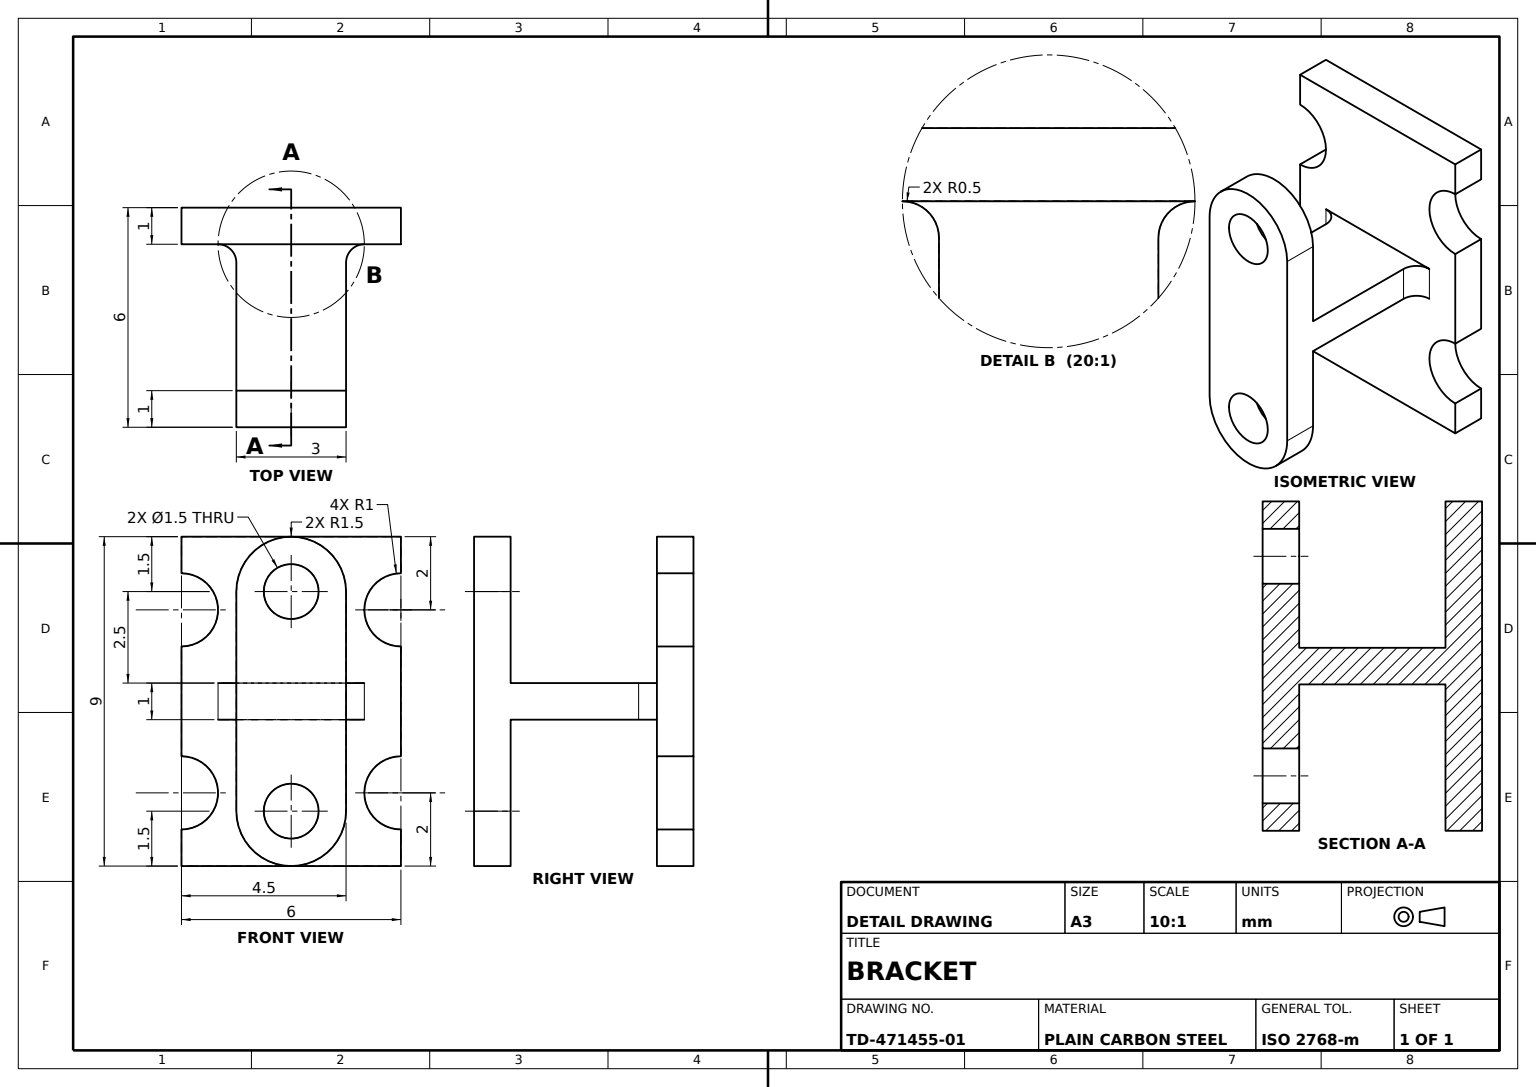
from build123d import *

# Parameters (mm, degrees)
BASE_PLATE_DEPTH   = 1
WEB_SKETCH_W       = 3
WEB_SKETCH_H       = 1
WEB_DEPTH          = 4
LUG_DEPTH          = 1
LUG_HOLES_SKETCH_R = 0.75
LUG_HOLES_2X_DEPTH = 1
WEB_FILLET_R0_5_R  = 0.5


with BuildPart() as part:
    # Base Plate Sketch → Base Plate (new body)
    with BuildSketch(Plane.XY):
        with BuildLine():
            Line((-3, 4.5), (3, 4.5))
            Line((3, 4.5), (3, 3.5))
            ThreePointArc((3, 3.5), (2, 2.5), (3, 1.5))
            Line((3, 1.5), (3, -1.5))
            ThreePointArc((3, -1.5), (2, -2.5), (3, -3.5))
            Line((3, -3.5), (3, -4.5))
            Line((3, -4.5), (-3, -4.5))
            Line((-3, -4.5), (-3, -3.5))
            ThreePointArc((-3, -3.5), (-2, -2.5), (-3, -1.5))
            Line((-3, -1.5), (-3, 1.5))
            ThreePointArc((-3, 1.5), (-2, 2.5), (-3, 3.5))
            Line((-3, 3.5), (-3, 4.5))
        make_face()
    extrude(amount=BASE_PLATE_DEPTH)

    # Web Sketch → Web (add)
    with BuildSketch(Plane.XY.offset(1)):
        Rectangle(WEB_SKETCH_W, WEB_SKETCH_H)
    extrude(amount=WEB_DEPTH)

    # Lug Sketch → Lug (add)
    with BuildSketch(Plane.XY.offset(5)):
        with BuildLine():
            Line((1.5, 3), (1.5, -3))
            ThreePointArc((1.5, -3), (0, -4.5), (-1.5, -3))
            Line((-1.5, -3), (-1.5, 3))
            ThreePointArc((-1.5, 3), (0, 4.5), (1.5, 3))
        make_face()
    extrude(amount=LUG_DEPTH)

    # Lug Holes Sketch → Lug Holes 2x (cut)
    with BuildSketch(Plane.XY.offset(6)):
        with Locations((0, 3)):
            Circle(LUG_HOLES_SKETCH_R)
        with Locations((0, -3)):
            Circle(LUG_HOLES_SKETCH_R)
    extrude(amount=-LUG_HOLES_2X_DEPTH, mode=Mode.SUBTRACT)

    # Web Fillet R0.5
    web_fillet_r0_5_edges = [part.edges().sort_by_distance(p)[0] for p in [
        (1.5, 0, 1),
        (-1.5, 0, 1),
    ]]
    fillet(web_fillet_r0_5_edges, radius=WEB_FILLET_R0_5_R)


solid = part.part
